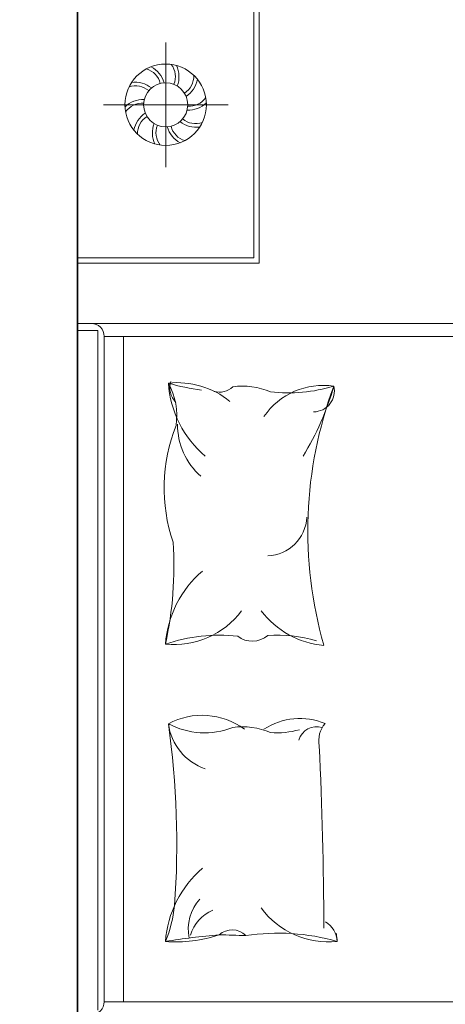
# Model space of a CAD drawing. Units: inches. Extents: x -638 to 186, y -762 to 59.
# Tile 6 of 31: x -164 to -140, y -511 to -457. Entities that reach past the tile are written whole.
import ezdxf

# ---------------------------------------------------------------- set-up
doc = ezdxf.new("R2010")
doc.units = ezdxf.units.IN
for name, color, linetype, lineweight in [('A-ANNO-DIMS', 2, 'Continuous', 18), ('furn', 8, 'Continuous', 13), ('wall', 7, 'Continuous', 35)]:
    doc.layers.add(name, color=color, linetype=linetype, lineweight=lineweight)
doc.styles.get("Standard").update_dxf_attribs({"font": 'arial.ttf'})
doc.dimstyles.new('ISO-25', dxfattribs={"dimtxt": 4, "dimasz": 4, "dimexe": 1.25, "dimexo": 0.625, "dimtad": 0, "dimlunit": 4, "dimtxsty": 'Standard', "dimcen": 2.5, "dimclrt": 256, "dimadec": 0, "dimazin": 0, "dimtfac": 1, "dimtmove": 0, "dimatfit": 3, "dimfxl": 1, "dimfxlon": 1, "dimarcsym": 0})

# ---------------------------------------------------------------- blocks, each defined once
blk = doc.blocks.new('BED-DOUBLE-WITH-NIGHTSTANDS')
for p, q in [((0, 59.951), (78.699, 59.951)), ((58.161, 59.951), (58.161, 58.826)), ((58.548, 11.244), (58.548, 59.951)), ((61.904, 59.951), (61.904, 49.874)), ((62.191, 59.951), (62.191, 50.162)), ((58.161, 58.826), (20.398, 58.826)), ((70.694, 51.596), (70.694, 58.516)), ((20.878, 58.468), (57.828, 58.468)), ((20.878, 58.468), (20.878, 13.164)), ((57.828, 13.164), (57.828, 58.468)), ((57.828, 57.404), (20.878, 57.404)), ((74.154, 55.056), (67.234, 55.056)), ((61.904, 49.874), (78.699, 49.874)), ((62.191, 50.162), (78.411, 50.162))]:
    blk.add_line(p, q)
for radius in [2.26, 1.225]:
    blk.add_circle((70.694, 55.056), radius)
for centre, radius, start, end in [((20.878, 59.188), 0.72, 180, 270), ((57.828, 59.188), 0.72, 270, 0), ((69.67, 56.366), 1.108, 355.462, 55.6998), ((69.537, 56.308), 1.452, 357.5103, 43.83), ((70.636, 56.718), 1.108, 319.462, 19.6998), ((70.494, 56.749), 1.452, 321.5103, 7.83), ((69.096, 55.514), 1.108, 31.462, 91.6998), ((69.022, 55.389), 1.452, 33.5103, 79.83), ((69.146, 54.343), 1.452, 69.5103, 115.83), ((71.623, 56.435), 1.108, 283.462, 343.6998), ((71.527, 56.544), 1.452, 285.5103, 331.83), ((69.132, 54.487), 1.108, 67.462, 127.6998), ((31.6, 54.462), 7.401, 175.3048, 198.6942), ((-14.535, 48.797), 39.263, 4.8098, 9.1892), ((26.929, 61.603), 7.073, 247.5178, 264.267), ((23.812, 49.204), 5.878, 40.4189, 85.9871), ((29.668, 101.849), 47.41, 265.8321, 278.0598), ((36.728, 51.85), 3.086, 97.7032, 160.9775), ((40.051, 52.903), 4.24, 151.7736, 201.6983), ((32.811, 53.035), 3.973, 323.7389, 28.1269), ((45.371, 54.589), 4.662, 174.11, 233.4289), ((45.094, 75.141), 20.542, 257.7438, 273.6284), ((40.322, 49.204), 5.878, 40.4189, 85.9871), ((32.161, 52.085), 9.076, 353.4947, 19.1867), ((49.42, 45.842), 9.304, 68.2026, 108.9817), ((55.647, 49.045), 5.878, 94.0129, 139.5811), ((53.423, 58.191), 3.75, 261.5958, 298.9092), ((54.987, 53.651), 1.175, 72.9226, 134.4009), ((50.598, 54.43), 4.662, 320.9404, 5.89), ((67.137, 51.406), 12.406, 163.6046, 172.3273), ((69.861, 53.569), 1.452, 105.5103, 151.83), ((69.765, 53.678), 1.108, 103.462, 163.6998), ((72.256, 55.625), 1.108, 247.462, 307.6998), ((52.894, 50.642), 3.752, 88.9577, 139.0518), ((70.894, 53.363), 1.452, 141.5103, 187.83), ((72.242, 55.77), 1.452, 249.5103, 295.83), ((24.909, 51.33), 2.472, 47.4509, 101.7793), ((23.874, 51.513), 2.284, 23.8756, 72.1383), ((70.753, 53.395), 1.108, 139.462, 199.6998), ((71.851, 53.804), 1.452, 177.5103, 223.83), ((71.718, 53.747), 1.108, 175.462, 235.6998), ((72.366, 54.723), 1.452, 213.5103, 259.83), ((72.292, 54.599), 1.108, 211.462, 271.6998), ((23.796, 51.371), 1.071, 314.4736, 42.1713), ((-32.064, 53.187), 56.669, 357.3905, 358.8876), ((55.833, 52.089), 1.101, 165.3506, 223.2684), ((32.112, 50.806), 4.034, 337.017, 7.5368), ((42.214, 50.25), 1.313, 142.0833, 220.902), ((51.033, 50.806), 4.034, 337.017, 7.5368), ((12.792, 48.807), 11.891, 344.0243, 8.7071), ((28.862, 46.013), 4.662, 126.5711, 185.89), ((40.21, 48.864), 4.4, 175.2233, 196.23), ((32.952, 47.606), 3.653, 337.4467, 33.0478), ((45.546, 45.855), 4.894, 127.1197, 175.09), ((33.322, 48.899), 7.916, 343.7954, 3.5554), ((47.91, 49.493), 2.28, 182.63, 266.884), ((51.147, 46.324), 3.96, 351.2621, 55.7572), ((63.68, 48.265), 8.986, 173.8296, 196.4356), ((35.105, 46.659), 1.047, 343.3521, 73.2995), ((47.026, 24.056), 23.109, 69.6507, 105.9631), ((59.196, 60.444), 15.291, 238.3499, 254.3137), ((24.019, 282.807), 236.536, 270.22759, 272.68343), ((35.378, 45.11), 1.447, 49.0991, 101.3702), ((54.788, 46.836), 1.147, 179.7727, 283.8018), ((24.141, 46.898), 1.366, 273.4709, 328.5412), ((23.812, 51.397), 5.878, 274.0129, 278.3417)]:
    blk.add_arc(centre, radius, start, end)
blk = doc.blocks.new('*D38')
at = {"layer": 'A-ANNO-DIMS', "color": 0, "lineweight": -2, "transparency": 16777216}
for p, q in [((182.663, -280.533), (184.913, -280.533)), ((183.663, -284.533), (183.663, -371.726)), ((183.663, -473.533), (183.663, -386.34)), ((182.663, -477.533), (184.913, -477.533))]:
    blk.add_line(p, q, dxfattribs=at)
at = {"layer": 'A-ANNO-DIMS', "color": 0, "lineweight": 30, "transparency": 16777216}
for points in [[(182.997, -284.533), (184.33, -284.533), (183.663, -280.533)], [(182.997, -473.533), (184.33, -473.533), (183.663, -477.533)]]:
    blk.add_solid(points, dxfattribs=at)
at = {"layer": 'Defpoints', "color": 0, "lineweight": 30, "transparency": 16777216}
for p in [(-404.526, -280.533), (-404.526, -477.533), (183.663, -477.533)]:
    blk.add_point(p, dxfattribs=at)
at = {"layer": 'A-ANNO-DIMS', "transparency": 16777216, "insert": (183.663, -379.033), "char_height": 4, "attachment_point": 5, "rotation": 90}
blk.add_mtext('16\'-5"', dxfattribs=at)

msp = doc.modelspace()

# ---------------------------------------------------------------- linework, layer by layer
at = {"layer": 'wall'}
msp.add_line((-160.526, -412.533), (-160.526, -539.033), dxfattribs=at)

# ---------------------------------------------------------------- block references
at = {"layer": 'furn', "rotation": 90.00000000000017}
msp.add_blockref('BED-DOUBLE-WITH-NIGHTSTANDS', (-100.575, -532.203), dxfattribs=at)

# ---------------------------------------------------------------- dimensions: what is measured, and where the dimension line sits
at = {"layer": 'A-ANNO-DIMS'}
dim = msp.add_linear_dim(base=(183.663, -477.533), p1=(-404.526, -280.533), p2=(-404.526, -477.533), angle=90, dimstyle='ISO-25', override={"dimdec": 1, "dimlfac": 1, "dimrnd": 0, "dimzin": 1, "dimdsep": 46, "dimlunit": 4, "dimfrac": 2}, dxfattribs=at)
dim.commit()
dim.dimension.update_dxf_attribs({"geometry": '*D38', "text_midpoint": (183.663, -379.033)})

doc.saveas('drawing.dxf')
